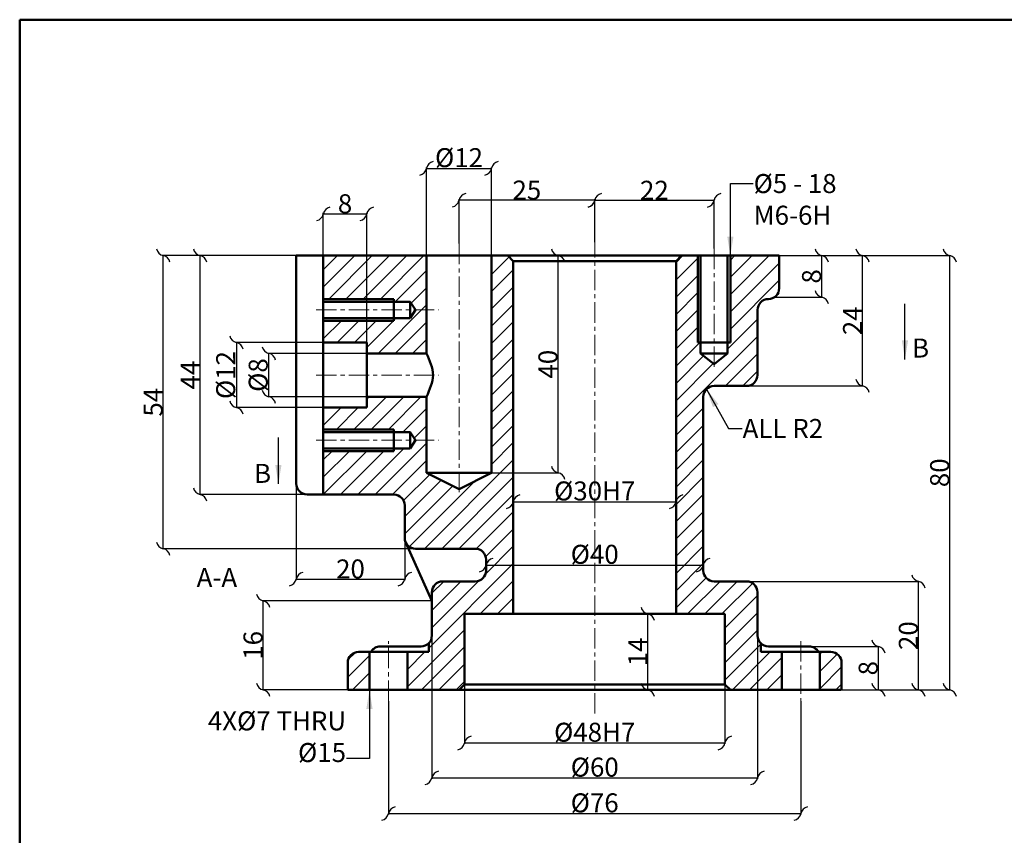
# Model space of a CAD drawing. Units: millimetres. Extents: x 10 to 373, y 9 to 285.
# Tile 2 of 3: x 10 to 191, y 135 to 285. Entities that reach past the tile are written whole.
import ezdxf

# ---------------------------------------------------------------- set-up
doc = ezdxf.new("R2010")
doc.units = ezdxf.units.MM
doc.header["$MEASUREMENT"] = 0
doc.linetypes.add('CENTER', pattern=[2, 1.25, -0.25, 0.25, -0.25])
for name, color, linetype, lineweight in [('M-CNTR', 1, 'CENTER', 18), ('M-DIMS', 2, 'Continuous', 25), ('M-HATC', 8, 'Continuous', 18), ('M-OUTL', 7, 'Continuous', 50), ('M-TEXT', 7, 'Continuous', 25), ('M-TTLB', 7, 'Continuous', 50)]:
    doc.layers.add(name, color=color, linetype=linetype, lineweight=lineweight)
doc.styles.get("Standard").update_dxf_attribs({"font": 'arial.ttf'})
doc.dimstyles.get("Standard").update_dxf_attribs({"dimtxt": 3.5, "dimasz": 3.5, "dimexe": 0.18, "dimexo": 0.0625, "dimgap": 0.09, "dimtad": 1, "dimdec": 0, "dimzin": 0, "dimdsep": 46, "dimtxsty": 'Standard', "dimblk": 'INTEGRAL', "dimcen": 0.09, "dimclre": 251, "dimadec": 0, "dimazin": 0, "dimtfac": 1, "dimtdec": 0, "dimtofl": 0, "dimtmove": 0, "dimatfit": 3, "dimfxl": 1, "dimtolj": 1, "dimtzin": 0, "dimarcsym": 0})

# ---------------------------------------------------------------- blocks, each defined once
blk = doc.blocks.new('_Integral')
at = {"color": 0, "linetype": 'ByBlock', "lineweight": -2}
for centre, start, end in [((0.445, -0.091), 102, 168), ((-0.445, 0.091), 282, 348)]:
    blk.add_arc(centre, 0.454, start, end, dxfattribs=at)
blk = doc.blocks.new('*D23')
at = {"layer": 'Defpoints', "color": 0, "transparency": 16777216}
for p in [(90.88, 252.1), (90.88, 244.06), (115.88, 244.35)]:
    blk.add_point(p, dxfattribs=at)
at = {"layer": 'M-DIMS', "color": 0, "lineweight": -2, "transparency": 16777216}
for p, q in [((90.88, 244.12), (90.88, 252.28)), ((115.88, 244.41), (115.88, 252.28)), ((115.88, 252.1), (90.88, 252.1))]:
    blk.add_line(p, q, dxfattribs=at)
at = {"layer": 'M-DIMS', "color": 0, "lineweight": -2, "transparency": 16777216, "xscale": 3.5, "yscale": 3.5, "zscale": 3.5, "rotation": 180}
blk.add_blockref('_Integral', (90.88, 252.1), dxfattribs=at)
at = {"layer": 'M-DIMS', "color": 0, "lineweight": -2, "transparency": 16777216, "xscale": 3.5, "yscale": 3.5, "zscale": 3.5}
blk.add_blockref('_Integral', (115.88, 252.1), dxfattribs=at)
at = {"layer": 'M-DIMS', "color": 0, "transparency": 16777216, "insert": (103.38, 253.98), "char_height": 3.5, "attachment_point": 5}
blk.add_mtext('\\A1;25', dxfattribs=at)
blk = doc.blocks.new('*D24')
at = {"layer": 'Defpoints', "color": 0, "transparency": 16777216}
for p in [(137.88, 252.09), (115.88, 244.35), (137.88, 243.16)]:
    blk.add_point(p, dxfattribs=at)
at = {"layer": 'M-DIMS', "color": 0, "lineweight": -2, "transparency": 16777216}
for p, q in [((115.88, 244.41), (115.88, 252.27)), ((137.88, 243.22), (137.88, 252.27)), ((115.88, 252.09), (137.88, 252.09))]:
    blk.add_line(p, q, dxfattribs=at)
at = {"layer": 'M-DIMS', "color": 0, "lineweight": -2, "transparency": 16777216, "xscale": 3.5, "yscale": 3.5, "zscale": 3.5, "rotation": 180}
blk.add_blockref('_Integral', (115.88, 252.09), dxfattribs=at)
at = {"layer": 'M-DIMS', "color": 0, "lineweight": -2, "transparency": 16777216, "xscale": 3.5, "yscale": 3.5, "zscale": 3.5}
blk.add_blockref('_Integral', (137.88, 252.09), dxfattribs=at)
at = {"layer": 'M-DIMS', "color": 0, "transparency": 16777216, "insert": (126.88, 253.94), "char_height": 3.5, "attachment_point": 5}
blk.add_mtext('\\A1;22', dxfattribs=at)
blk = doc.blocks.new('*D25')
at = {"layer": 'Defpoints', "color": 0, "transparency": 16777216}
for p in [(96.88, 257.98), (84.88, 241.9), (96.88, 241.9)]:
    blk.add_point(p, dxfattribs=at)
at = {"layer": 'M-DIMS', "color": 0, "lineweight": -2, "transparency": 16777216}
for p, q in [((84.88, 241.96), (84.88, 258.16)), ((84.88, 257.98), (96.88, 257.98)), ((96.88, 241.96), (96.88, 258.16))]:
    blk.add_line(p, q, dxfattribs=at)
at = {"layer": 'M-DIMS', "color": 0, "lineweight": -2, "transparency": 16777216, "xscale": 3.5, "yscale": 3.5, "zscale": 3.5, "rotation": 180}
blk.add_blockref('_Integral', (84.88, 257.98), dxfattribs=at)
at = {"layer": 'M-DIMS', "color": 0, "lineweight": -2, "transparency": 16777216, "xscale": 3.5, "yscale": 3.5, "zscale": 3.5}
blk.add_blockref('_Integral', (96.88, 257.98), dxfattribs=at)
at = {"layer": 'M-DIMS', "color": 0, "transparency": 16777216, "insert": (90.88, 259.95), "char_height": 3.5, "attachment_point": 5}
blk.add_mtext('\\A1;%%C12', dxfattribs=at)
blk = doc.blocks.new('*D26')
at = {"layer": 'Defpoints', "color": 0, "transparency": 16777216}
for p in [(73.88, 249.58), (65.88, 241.9), (73.88, 225.9)]:
    blk.add_point(p, dxfattribs=at)
at = {"layer": 'M-DIMS', "color": 0, "lineweight": -2, "transparency": 16777216}
for p, q in [((65.88, 241.96), (65.88, 249.76)), ((65.88, 249.58), (73.88, 249.58)), ((73.88, 225.96), (73.88, 249.76))]:
    blk.add_line(p, q, dxfattribs=at)
at = {"layer": 'M-DIMS', "color": 0, "lineweight": -2, "transparency": 16777216, "xscale": 3.5, "yscale": 3.5, "zscale": 3.5, "rotation": 180}
blk.add_blockref('_Integral', (65.88, 249.58), dxfattribs=at)
at = {"layer": 'M-DIMS', "color": 0, "lineweight": -2, "transparency": 16777216, "xscale": 3.5, "yscale": 3.5, "zscale": 3.5}
blk.add_blockref('_Integral', (73.88, 249.58), dxfattribs=at)
at = {"layer": 'M-DIMS', "color": 0, "transparency": 16777216, "insert": (69.88, 251.46), "char_height": 3.5, "attachment_point": 5}
blk.add_mtext('\\A1;8', dxfattribs=at)
blk = doc.blocks.new('*D27')
at = {"layer": 'Defpoints', "color": 0, "transparency": 16777216}
for p in [(55.86, 223.9), (73.88, 223.9), (73.88, 215.9)]:
    blk.add_point(p, dxfattribs=at)
at = {"layer": 'M-DIMS', "color": 0, "lineweight": -2, "transparency": 16777216}
for p, q in [((73.82, 223.9), (55.68, 223.9)), ((55.86, 215.9), (55.86, 223.9)), ((73.82, 215.9), (55.68, 215.9))]:
    blk.add_line(p, q, dxfattribs=at)
at = {"layer": 'M-DIMS', "color": 0, "lineweight": -2, "transparency": 16777216, "xscale": 3.5, "yscale": 3.5, "zscale": 3.5}
for p, rotation in [((55.86, 223.9), 90), ((55.86, 215.9), 270)]:
    blk.add_blockref('_Integral', p, dxfattribs=dict(at, rotation=rotation))
at = {"layer": 'M-DIMS', "color": 0, "transparency": 16777216, "insert": (53.88, 219.9), "char_height": 3.5, "attachment_point": 5, "rotation": 90}
blk.add_mtext('\\A1;%%C8', dxfattribs=at)
blk = doc.blocks.new('*D28')
at = {"layer": 'Defpoints', "color": 0, "transparency": 16777216}
for p in [(65.88, 225.9), (49.87, 213.9), (65.88, 213.9)]:
    blk.add_point(p, dxfattribs=at)
at = {"layer": 'M-DIMS', "color": 0, "lineweight": -2, "transparency": 16777216}
for p, q in [((65.82, 225.9), (49.69, 225.9)), ((49.87, 225.9), (49.87, 213.9)), ((65.82, 213.9), (49.69, 213.9))]:
    blk.add_line(p, q, dxfattribs=at)
at = {"layer": 'M-DIMS', "color": 0, "lineweight": -2, "transparency": 16777216, "xscale": 3.5, "yscale": 3.5, "zscale": 3.5}
for p, rotation in [((49.87, 225.9), 90), ((49.87, 213.9), 270)]:
    blk.add_blockref('_Integral', p, dxfattribs=dict(at, rotation=rotation))
at = {"layer": 'M-DIMS', "color": 0, "transparency": 16777216, "insert": (47.89, 219.9), "char_height": 3.5, "attachment_point": 5, "rotation": 90}
blk.add_mtext('\\A1;%%C12', dxfattribs=at)
blk = doc.blocks.new('*D29')
at = {"layer": 'Defpoints', "color": 0, "transparency": 16777216}
for p in [(43.17, 241.9), (60.88, 241.9), (62.88, 197.9)]:
    blk.add_point(p, dxfattribs=at)
at = {"layer": 'M-DIMS', "color": 0, "lineweight": -2, "transparency": 16777216}
for p, q in [((60.82, 241.9), (42.99, 241.9)), ((43.17, 197.9), (43.17, 241.9)), ((62.82, 197.9), (42.99, 197.9))]:
    blk.add_line(p, q, dxfattribs=at)
at = {"layer": 'M-DIMS', "color": 0, "lineweight": -2, "transparency": 16777216, "xscale": 3.5, "yscale": 3.5, "zscale": 3.5}
for p, rotation in [((43.17, 241.9), 90), ((43.17, 197.9), 270)]:
    blk.add_blockref('_Integral', p, dxfattribs=dict(at, rotation=rotation))
at = {"layer": 'M-DIMS', "color": 0, "transparency": 16777216, "insert": (41.33, 219.9), "char_height": 3.5, "attachment_point": 5, "rotation": 90}
blk.add_mtext('\\A1;44', dxfattribs=at)
blk = doc.blocks.new('*D30')
at = {"layer": 'Defpoints', "color": 0, "transparency": 16777216}
for p in [(36.39, 241.9), (60.88, 241.9), (82.88, 187.9)]:
    blk.add_point(p, dxfattribs=at)
at = {"layer": 'M-DIMS', "color": 0, "lineweight": -2, "transparency": 16777216}
for p, q in [((60.82, 241.9), (36.21, 241.9)), ((36.39, 187.9), (36.39, 241.9)), ((82.82, 187.9), (36.21, 187.9))]:
    blk.add_line(p, q, dxfattribs=at)
at = {"layer": 'M-DIMS', "color": 0, "lineweight": -2, "transparency": 16777216, "xscale": 3.5, "yscale": 3.5, "zscale": 3.5}
for p, rotation in [((36.39, 241.9), 90), ((36.39, 187.9), 270)]:
    blk.add_blockref('_Integral', p, dxfattribs=dict(at, rotation=rotation))
at = {"layer": 'M-DIMS', "color": 0, "transparency": 16777216, "insert": (34.52, 214.9), "char_height": 3.5, "attachment_point": 5, "rotation": 90}
blk.add_mtext('\\A1;54', dxfattribs=at)
blk = doc.blocks.new('*D31')
at = {"layer": 'Defpoints', "color": 0, "transparency": 16777216}
for p in [(60.88, 199.9), (80.88, 189.9), (80.88, 182.31)]:
    blk.add_point(p, dxfattribs=at)
at = {"layer": 'M-DIMS', "color": 0, "lineweight": -2, "transparency": 16777216}
for p, q in [((60.88, 199.84), (60.88, 182.13)), ((80.88, 189.84), (80.88, 182.13)), ((60.88, 182.31), (80.88, 182.31))]:
    blk.add_line(p, q, dxfattribs=at)
at = {"layer": 'M-DIMS', "color": 0, "lineweight": -2, "transparency": 16777216, "xscale": 3.5, "yscale": 3.5, "zscale": 3.5, "rotation": 180}
blk.add_blockref('_Integral', (60.88, 182.31), dxfattribs=at)
at = {"layer": 'M-DIMS', "color": 0, "lineweight": -2, "transparency": 16777216, "xscale": 3.5, "yscale": 3.5, "zscale": 3.5}
blk.add_blockref('_Integral', (80.88, 182.31), dxfattribs=at)
at = {"layer": 'M-DIMS', "color": 0, "transparency": 16777216, "insert": (70.88, 184.18), "char_height": 3.5, "attachment_point": 5}
blk.add_mtext('\\A1;20', dxfattribs=at)
blk = doc.blocks.new('*D32')
at = {"layer": 'Defpoints', "color": 0, "transparency": 16777216}
for p in [(54.8, 178.31), (85.88, 178.31), (70.38, 161.9)]:
    blk.add_point(p, dxfattribs=at)
at = {"layer": 'M-DIMS', "color": 0, "lineweight": -2, "transparency": 16777216}
for p, q in [((85.82, 178.31), (54.62, 178.31)), ((54.8, 161.9), (54.8, 178.31)), ((70.32, 161.9), (54.62, 161.9))]:
    blk.add_line(p, q, dxfattribs=at)
at = {"layer": 'M-DIMS', "color": 0, "lineweight": -2, "transparency": 16777216, "xscale": 3.5, "yscale": 3.5, "zscale": 3.5}
for p, rotation in [((54.8, 178.31), 90), ((54.8, 161.9), 270)]:
    blk.add_blockref('_Integral', p, dxfattribs=dict(at, rotation=rotation))
at = {"layer": 'M-DIMS', "color": 0, "transparency": 16777216, "insert": (52.92, 170.1), "char_height": 3.5, "attachment_point": 5, "rotation": 90}
blk.add_mtext('\\A1;16', dxfattribs=at)
blk = doc.blocks.new('*D33')
at = {"layer": 'Defpoints', "color": 0, "transparency": 16777216}
for p in [(149.88, 241.9), (157.72, 241.9), (149.01, 234.25)]:
    blk.add_point(p, dxfattribs=at)
at = {"layer": 'M-DIMS', "color": 0, "lineweight": -2, "transparency": 16777216}
for p, q in [((149.95, 241.9), (157.9, 241.9)), ((157.72, 234.25), (157.72, 241.9)), ((149.08, 234.25), (157.9, 234.25))]:
    blk.add_line(p, q, dxfattribs=at)
at = {"layer": 'M-DIMS', "color": 0, "lineweight": -2, "transparency": 16777216, "xscale": 3.5, "yscale": 3.5, "zscale": 3.5}
for p, rotation in [((157.72, 241.9), 90), ((157.72, 234.25), 270)]:
    blk.add_blockref('_Integral', p, dxfattribs=dict(at, rotation=rotation))
at = {"layer": 'M-DIMS', "color": 0, "transparency": 16777216, "insert": (155.84, 238.08), "char_height": 3.5, "attachment_point": 5, "rotation": 90}
blk.add_mtext('\\A1;8', dxfattribs=at)
blk = doc.blocks.new('*D34')
at = {"layer": 'Defpoints', "color": 0, "transparency": 16777216}
for p in [(149.88, 241.9), (165.24, 241.9), (143.88, 217.9)]:
    blk.add_point(p, dxfattribs=at)
at = {"layer": 'M-DIMS', "color": 0, "lineweight": -2, "transparency": 16777216}
for p, q in [((149.95, 241.9), (165.42, 241.9)), ((165.24, 217.9), (165.24, 241.9)), ((143.95, 217.9), (165.42, 217.9))]:
    blk.add_line(p, q, dxfattribs=at)
at = {"layer": 'M-DIMS', "color": 0, "lineweight": -2, "transparency": 16777216, "xscale": 3.5, "yscale": 3.5, "zscale": 3.5}
for p, rotation in [((165.24, 241.9), 90), ((165.24, 217.9), 270)]:
    blk.add_blockref('_Integral', p, dxfattribs=dict(at, rotation=rotation))
at = {"layer": 'M-DIMS', "color": 0, "transparency": 16777216, "insert": (163.39, 229.9), "char_height": 3.5, "attachment_point": 5, "rotation": 90}
blk.add_mtext('\\A1;24', dxfattribs=at)
blk = doc.blocks.new('*D35')
at = {"layer": 'Defpoints', "color": 0, "transparency": 16777216}
for p in [(155.38, 169.9), (168.15, 169.9), (161.38, 161.9)]:
    blk.add_point(p, dxfattribs=at)
at = {"layer": 'M-DIMS', "color": 0, "lineweight": -2, "transparency": 16777216}
for p, q in [((155.45, 169.9), (168.33, 169.9)), ((168.15, 161.9), (168.15, 169.9)), ((161.45, 161.9), (168.33, 161.9))]:
    blk.add_line(p, q, dxfattribs=at)
at = {"layer": 'M-DIMS', "color": 0, "lineweight": -2, "transparency": 16777216, "xscale": 3.5, "yscale": 3.5, "zscale": 3.5}
for p, rotation in [((168.15, 169.9), 90), ((168.15, 161.9), 270)]:
    blk.add_blockref('_Integral', p, dxfattribs=dict(at, rotation=rotation))
at = {"layer": 'M-DIMS', "color": 0, "transparency": 16777216, "insert": (166.27, 165.9), "char_height": 3.5, "attachment_point": 5, "rotation": 90}
blk.add_mtext('\\A1;8', dxfattribs=at)
blk = doc.blocks.new('*D36')
at = {"layer": 'Defpoints', "color": 0, "transparency": 16777216}
for p in [(137.88, 181.9), (175.54, 181.9), (161.38, 161.9)]:
    blk.add_point(p, dxfattribs=at)
at = {"layer": 'M-DIMS', "color": 0, "lineweight": -2, "transparency": 16777216}
for p, q in [((137.95, 181.9), (175.72, 181.9)), ((175.54, 161.9), (175.54, 181.9)), ((161.45, 161.9), (175.72, 161.9))]:
    blk.add_line(p, q, dxfattribs=at)
at = {"layer": 'M-DIMS', "color": 0, "lineweight": -2, "transparency": 16777216, "xscale": 3.5, "yscale": 3.5, "zscale": 3.5}
for p, rotation in [((175.54, 181.9), 90), ((175.54, 161.9), 270)]:
    blk.add_blockref('_Integral', p, dxfattribs=dict(at, rotation=rotation))
at = {"layer": 'M-DIMS', "color": 0, "transparency": 16777216, "insert": (173.67, 171.9), "char_height": 3.5, "attachment_point": 5, "rotation": 90}
blk.add_mtext('\\A1;20', dxfattribs=at)
blk = doc.blocks.new('*D37')
at = {"layer": 'Defpoints', "color": 0, "transparency": 16777216}
for p in [(149.88, 241.9), (181.31, 241.9), (161.38, 161.9)]:
    blk.add_point(p, dxfattribs=at)
at = {"layer": 'M-DIMS', "color": 0, "lineweight": -2, "transparency": 16777216}
for p, q in [((149.95, 241.9), (181.49, 241.9)), ((181.31, 161.9), (181.31, 241.9)), ((161.45, 161.9), (181.49, 161.9))]:
    blk.add_line(p, q, dxfattribs=at)
at = {"layer": 'M-DIMS', "color": 0, "lineweight": -2, "transparency": 16777216, "xscale": 3.5, "yscale": 3.5, "zscale": 3.5}
for p, rotation in [((181.31, 241.9), 90), ((181.31, 161.9), 270)]:
    blk.add_blockref('_Integral', p, dxfattribs=dict(at, rotation=rotation))
at = {"layer": 'M-DIMS', "color": 0, "transparency": 16777216, "insert": (179.44, 201.9), "char_height": 3.5, "attachment_point": 5, "rotation": 90}
blk.add_mtext('\\A1;80', dxfattribs=at)
blk = doc.blocks.new('*D38')
at = {"layer": 'Defpoints', "color": 0, "transparency": 16777216}
for p in [(125.66, 175.9), (125.66, 175.9), (125.66, 161.9)]:
    blk.add_point(p, dxfattribs=at)
at = {"layer": 'M-DIMS', "color": 0, "lineweight": -2, "transparency": 16777216}
for p, q in [((125.66, 161.9), (125.66, 175.9)), ((125.72, 175.9), (125.84, 175.9)), ((125.72, 161.9), (125.84, 161.9))]:
    blk.add_line(p, q, dxfattribs=at)
at = {"layer": 'M-DIMS', "color": 0, "lineweight": -2, "transparency": 16777216, "xscale": 3.5, "yscale": 3.5, "zscale": 3.5}
for p, rotation in [((125.66, 175.9), 90), ((125.66, 161.9), 270)]:
    blk.add_blockref('_Integral', p, dxfattribs=dict(at, rotation=rotation))
at = {"layer": 'M-DIMS', "color": 0, "transparency": 16777216, "insert": (123.81, 168.9), "char_height": 3.5, "attachment_point": 5, "rotation": 90}
blk.add_mtext('\\A1;14', dxfattribs=at)
blk = doc.blocks.new('*D39')
at = {"layer": 'Defpoints', "color": 0, "transparency": 16777216}
for p in [(91.88, 162.9), (139.88, 162.9), (139.88, 152.12)]:
    blk.add_point(p, dxfattribs=at)
at = {"layer": 'M-DIMS', "color": 0, "lineweight": -2, "transparency": 16777216}
for p, q in [((91.88, 162.84), (91.88, 151.94)), ((139.88, 162.84), (139.88, 151.94)), ((91.88, 152.12), (139.88, 152.12))]:
    blk.add_line(p, q, dxfattribs=at)
at = {"layer": 'M-DIMS', "color": 0, "lineweight": -2, "transparency": 16777216, "xscale": 3.5, "yscale": 3.5, "zscale": 3.5, "rotation": 180}
blk.add_blockref('_Integral', (91.88, 152.12), dxfattribs=at)
at = {"layer": 'M-DIMS', "color": 0, "lineweight": -2, "transparency": 16777216, "xscale": 3.5, "yscale": 3.5, "zscale": 3.5}
blk.add_blockref('_Integral', (139.88, 152.12), dxfattribs=at)
at = {"layer": 'M-DIMS', "color": 0, "transparency": 16777216, "insert": (115.88, 154.1), "char_height": 3.5, "attachment_point": 5}
blk.add_mtext('\\A1;%%C48H7', dxfattribs=at)
blk = doc.blocks.new('*D40')
at = {"layer": 'Defpoints', "color": 0, "transparency": 16777216}
for p in [(85.88, 171.9), (145.89, 171.81), (145.89, 145.69)]:
    blk.add_point(p, dxfattribs=at)
at = {"layer": 'M-DIMS', "color": 0, "lineweight": -2, "transparency": 16777216}
for p, q in [((85.88, 171.84), (85.88, 145.51)), ((145.89, 171.74), (145.89, 145.51)), ((85.88, 145.69), (145.89, 145.69))]:
    blk.add_line(p, q, dxfattribs=at)
at = {"layer": 'M-DIMS', "color": 0, "lineweight": -2, "transparency": 16777216, "xscale": 3.5, "yscale": 3.5, "zscale": 3.5, "rotation": 180}
blk.add_blockref('_Integral', (85.88, 145.69), dxfattribs=at)
at = {"layer": 'M-DIMS', "color": 0, "lineweight": -2, "transparency": 16777216, "xscale": 3.5, "yscale": 3.5, "zscale": 3.5}
blk.add_blockref('_Integral', (145.89, 145.69), dxfattribs=at)
at = {"layer": 'M-DIMS', "color": 0, "transparency": 16777216, "insert": (115.89, 147.67), "char_height": 3.5, "attachment_point": 5}
blk.add_mtext('\\A1;%%C60', dxfattribs=at)
blk = doc.blocks.new('*D41')
at = {"layer": 'Defpoints', "color": 0, "transparency": 16777216}
for p in [(77.88, 159.9), (153.88, 159.9), (153.88, 139.12)]:
    blk.add_point(p, dxfattribs=at)
at = {"layer": 'M-DIMS', "color": 0, "lineweight": -2, "transparency": 16777216}
for p, q in [((77.88, 159.84), (77.88, 138.94)), ((153.88, 159.84), (153.88, 138.94)), ((77.88, 139.12), (153.88, 139.12))]:
    blk.add_line(p, q, dxfattribs=at)
at = {"layer": 'M-DIMS', "color": 0, "lineweight": -2, "transparency": 16777216, "xscale": 3.5, "yscale": 3.5, "zscale": 3.5, "rotation": 180}
blk.add_blockref('_Integral', (77.88, 139.12), dxfattribs=at)
at = {"layer": 'M-DIMS', "color": 0, "lineweight": -2, "transparency": 16777216, "xscale": 3.5, "yscale": 3.5, "zscale": 3.5}
blk.add_blockref('_Integral', (153.88, 139.12), dxfattribs=at)
at = {"layer": 'M-DIMS', "color": 0, "transparency": 16777216, "insert": (115.88, 141.09), "char_height": 3.5, "attachment_point": 5}
blk.add_mtext('\\A1;%%C76', dxfattribs=at)
blk = doc.blocks.new('*D42')
at = {"layer": 'Defpoints', "color": 0, "transparency": 16777216}
for p in [(109.14, 241.9), (109.15, 241.9), (96.88, 201.9)]:
    blk.add_point(p, dxfattribs=at)
at = {"layer": 'M-DIMS', "color": 0, "lineweight": -2, "transparency": 16777216}
for p, q in [((109.15, 201.9), (109.15, 241.9)), ((109.2, 241.9), (109.33, 241.9)), ((96.95, 201.9), (109.33, 201.9))]:
    blk.add_line(p, q, dxfattribs=at)
at = {"layer": 'M-DIMS', "color": 0, "lineweight": -2, "transparency": 16777216, "xscale": 3.5, "yscale": 3.5, "zscale": 3.5}
for p, rotation in [((109.15, 241.9), 90), ((109.15, 201.9), 270)]:
    blk.add_blockref('_Integral', p, dxfattribs=dict(at, rotation=rotation))
at = {"layer": 'M-DIMS', "color": 0, "transparency": 16777216, "insert": (107.27, 221.9), "char_height": 3.5, "attachment_point": 5, "rotation": 90}
blk.add_mtext('\\A1;40', dxfattribs=at)
blk = doc.blocks.new('*D43')
at = {"layer": 'Defpoints', "color": 0, "transparency": 16777216}
for p in [(100.88, 196.57), (130.88, 196.57), (130.88, 196.57)]:
    blk.add_point(p, dxfattribs=at)
at = {"layer": 'M-DIMS', "color": 0, "lineweight": -2, "transparency": 16777216}
for p, q in [((100.88, 196.63), (100.88, 196.75)), ((100.88, 196.57), (130.88, 196.57)), ((130.88, 196.63), (130.88, 196.75))]:
    blk.add_line(p, q, dxfattribs=at)
at = {"layer": 'M-DIMS', "color": 0, "lineweight": -2, "transparency": 16777216, "xscale": 3.5, "yscale": 3.5, "zscale": 3.5, "rotation": 180}
blk.add_blockref('_Integral', (100.88, 196.57), dxfattribs=at)
at = {"layer": 'M-DIMS', "color": 0, "lineweight": -2, "transparency": 16777216, "xscale": 3.5, "yscale": 3.5, "zscale": 3.5}
blk.add_blockref('_Integral', (130.88, 196.57), dxfattribs=at)
at = {"layer": 'M-DIMS', "color": 0, "transparency": 16777216, "insert": (115.88, 198.55), "char_height": 3.5, "attachment_point": 5}
blk.add_mtext('\\A1;%%C30H7', dxfattribs=at)
blk = doc.blocks.new('*D44')
at = {"layer": 'Defpoints', "color": 0, "transparency": 16777216}
for p in [(95.88, 184.9), (135.88, 184.9), (135.88, 184.9)]:
    blk.add_point(p, dxfattribs=at)
at = {"layer": 'M-DIMS', "color": 0, "lineweight": -2, "transparency": 16777216}
for p, q in [((95.88, 184.96), (95.88, 185.08)), ((135.88, 184.96), (135.88, 185.08)), ((95.88, 184.9), (135.88, 184.9))]:
    blk.add_line(p, q, dxfattribs=at)
at = {"layer": 'M-DIMS', "color": 0, "lineweight": -2, "transparency": 16777216, "xscale": 3.5, "yscale": 3.5, "zscale": 3.5, "rotation": 180}
blk.add_blockref('_Integral', (95.88, 184.9), dxfattribs=at)
at = {"layer": 'M-DIMS', "color": 0, "lineweight": -2, "transparency": 16777216, "xscale": 3.5, "yscale": 3.5, "zscale": 3.5}
blk.add_blockref('_Integral', (135.88, 184.9), dxfattribs=at)
at = {"layer": 'M-DIMS', "color": 0, "transparency": 16777216, "insert": (115.88, 186.88), "char_height": 3.5, "attachment_point": 5}
blk.add_mtext('\\A1;%%C40', dxfattribs=at)
blk = doc.blocks.new('TAPPED-HOLE-M6')
for p, q in [((0, 4), (13, 4)), ((13, 0), (13, 4)), ((0, 3.5), (16, 3.5)), ((16, 0.5), (16, 3.5)), ((17, 2), (16, 3.5)), ((16, 0.5), (17, 2)), ((0, 0.5), (16, 0.5)), ((0, 0), (13, 0))]:
    blk.add_line(p, q)

msp = doc.modelspace()

# ---------------------------------------------------------------- hatches: boundary and pattern name
at = {"layer": 'M-HATC'}
h = msp.add_hatch(dxfattribs=at)
h.set_pattern_fill('ANSI31', color=256, scale=18)
h.set_pattern_definition([(45, (-376.4816, -107.6296), (-1.59099, 1.59099), [])])
h.paths.add_polyline_path([(84.88, 241.9), (65.88, 241.9), (65.88, 233.9), (78.88, 233.9), (78.88, 233.4), (81.88, 233.4), (82.88, 231.9), (84.88, 231.9)])
h.paths.add_polyline_path([(84.88, 231.9), (82.88, 231.9), (81.88, 230.4), (78.88, 230.4), (78.88, 229.9), (65.88, 229.9), (65.88, 225.9), (73.88, 225.9), (73.88, 223.9), (84.88, 223.9)])
h.paths.add_polyline_path([(84.88, 215.9), (73.88, 215.9), (73.88, 213.9), (65.88, 213.9), (65.88, 209.9), (78.88, 209.9), (78.88, 209.4), (81.88, 209.4), (82.88, 207.9), (84.88, 207.9)], flags=17)
h.paths.add_polyline_path([(90.88, 198.9), (84.88, 201.9), (84.88, 207.9), (82.88, 207.9), (81.88, 206.4), (78.88, 206.4), (78.88, 205.9), (65.88, 205.9), (65.88, 197.9), (78.88, 197.9, -0.414214), (80.88, 195.9), (80.88, 189.9, 0.414214), (82.88, 187.9), (93.88, 187.9, -0.414214), (95.88, 185.9), (95.88, 183.9, -0.414214), (93.88, 181.9), (87.88, 181.9, 0.414214), (85.88, 179.9), (85.88, 171.9, -0.198912), (85.3, 170.49), (85.3, 168.9), (81.38, 168.9), (81.38, 161.9), (90.88, 161.9), (91.88, 162.9), (91.88, 175.9), (100.88, 175.9), (100.88, 240.9), (99.88, 241.9), (96.88, 241.9), (96.88, 201.9)])
h.paths.add_polyline_path([(150.38, 168.9), (146.47, 168.9), (146.47, 170.49, -0.198912), (145.88, 171.9), (145.88, 179.9, 0.414214), (143.88, 181.9), (137.88, 181.9, -0.414214), (135.88, 183.9), (135.88, 215.9, -0.414214), (137.88, 217.9), (143.88, 217.9, 0.414214), (145.88, 219.9), (145.88, 231.9, -0.414214), (147.88, 233.9, 0.414214), (149.88, 235.9), (149.88, 241.9), (140.88, 241.9), (140.88, 225.9), (140.38, 225.9), (140.38, 223.9), (137.88, 221.9), (135.38, 223.9), (135.38, 225.9), (134.88, 225.9), (134.88, 241.9), (131.88, 241.9), (130.88, 240.9), (130.88, 175.9), (139.88, 175.9), (139.88, 162.9), (140.88, 161.9), (150.38, 161.9)])
edge = h.paths.add_edge_path()
edge.add_arc((72.38, 166.9), 2, 90, 180)
edge.add_line((70.38, 166.9), (70.38, 161.9))
edge.add_line((70.38, 161.9), (74.38, 161.9))
edge.add_line((74.38, 161.9), (74.38, 168.9))
edge.add_line((74.38, 168.9), (72.38, 168.9))
edge = h.paths.add_edge_path()
edge.add_arc((159.38, 166.9), 2, 360, 450)
edge.add_line((159.38, 168.9), (157.38, 168.9))
edge.add_line((157.38, 168.9), (157.38, 161.9))
edge.add_line((157.38, 161.9), (161.38, 161.9))
edge.add_line((161.38, 161.9), (161.38, 166.9))

# ---------------------------------------------------------------- linework, layer by layer
at = {"layer": 'M-CNTR', "ltscale": 3}
for p, q in [((90.88, 244.06), (90.88, 197.49)), ((115.88, 157.55), (115.88, 244.35)), ((137.88, 243.16), (137.88, 221.41)), ((64.57, 231.9), (87.14, 231.9)), ((64.57, 219.9), (87.14, 219.9)), ((64.57, 207.9), (87.14, 207.9)), ((77.88, 159.9), (77.88, 170.9)), ((153.88, 170.9), (153.88, 159.9))]:
    msp.add_line(p, q, dxfattribs=at)
at = {"layer": 'M-OUTL'}
for p, q in [((60.88, 241.9), (149.88, 241.9)), ((60.88, 241.9), (60.88, 199.9)), ((65.88, 197.9), (65.88, 241.9)), ((84.88, 223.9), (84.88, 241.9)), ((96.88, 201.9), (96.88, 241.9)), ((99.88, 241.9), (100.88, 240.9)), ((130.88, 240.9), (131.88, 241.9)), ((134.88, 241.9), (134.88, 225.9)), ((135.38, 241.9), (135.38, 223.9)), ((140.38, 241.9), (140.38, 223.9)), ((140.88, 241.9), (140.88, 225.9)), ((149.88, 241.9), (149.88, 235.9)), ((100.88, 175.9), (100.88, 240.9)), ((100.88, 240.9), (130.88, 240.9)), ((130.88, 175.9), (130.88, 240.9)), ((147.88, 233.9), (147.88, 233.9)), ((145.88, 219.9), (145.88, 231.9)), ((65.88, 225.9), (73.88, 225.9)), ((73.88, 213.9), (73.88, 225.9)), ((134.88, 225.9), (140.88, 225.9)), ((73.88, 223.9), (84.88, 223.9)), ((135.38, 223.9), (140.38, 223.9)), ((135.38, 223.9), (137.88, 221.9)), ((137.88, 221.9), (140.38, 223.9)), ((137.88, 217.9), (143.88, 217.9)), ((73.88, 215.9), (84.88, 215.9)), ((84.88, 201.9), (84.88, 215.9)), ((135.88, 183.9), (135.88, 215.9)), ((65.88, 213.9), (73.88, 213.9)), ((84.88, 201.9), (96.88, 201.9)), ((84.88, 201.9), (90.88, 198.9)), ((90.88, 198.9), (96.88, 201.9)), ((62.88, 197.9), (78.88, 197.9)), ((80.88, 195.9), (80.88, 189.9)), ((85.88, 178.31), (81.11, 188.97)), ((82.88, 187.9), (93.88, 187.9)), ((95.88, 183.9), (95.88, 185.9)), ((93.88, 181.9), (87.88, 181.9)), ((137.88, 181.9), (143.88, 181.9)), ((85.88, 171.9), (85.88, 179.9)), ((145.88, 179.9), (145.88, 171.9)), ((91.88, 162.9), (91.88, 175.9)), ((91.88, 175.9), (139.88, 175.9)), ((139.88, 162.9), (139.88, 175.9)), ((72.38, 168.9), (85.3, 168.9)), ((74.38, 161.9), (74.38, 168.9)), ((76.38, 169.9), (83.88, 169.9)), ((81.38, 161.9), (81.38, 168.9)), ((85.3, 170.49), (85.3, 168.9)), ((146.47, 170.49), (146.47, 168.9)), ((146.47, 168.9), (159.38, 168.9)), ((155.38, 169.9), (147.88, 169.9)), ((150.38, 168.9), (150.38, 161.9)), ((157.38, 168.9), (157.38, 161.9)), ((70.38, 161.9), (70.38, 166.9)), ((161.38, 161.9), (161.38, 166.9)), ((70.38, 161.9), (161.38, 161.9)), ((90.88, 161.9), (91.88, 162.9)), ((91.88, 162.9), (139.88, 162.9)), ((139.88, 162.9), (140.88, 161.9))]:
    msp.add_line(p, q, dxfattribs=at)
for centre, start, end in [((147.88, 235.9), 270, 0), ((147.88, 231.9), 90, 180), ((143.88, 219.9), 270, 0), ((137.88, 215.9), 90, 180), ((62.88, 199.9), 180, 270), ((78.88, 195.9), 0, 90), ((82.88, 189.9), 180, 270), ((93.88, 185.9), 0, 90), ((93.88, 183.9), 270, 0), ((137.88, 183.9), 180, 270), ((87.88, 179.9), 90, 180), ((143.88, 179.9), 0, 90), ((83.88, 171.9), 270, 0), ((147.88, 171.9), 180, 270), ((72.38, 166.9), 90, 180), ((76.38, 167.9), 90, 150), ((155.38, 167.9), 30, 90), ((159.38, 166.9), 0, 90)]:
    msp.add_arc(centre, 2, start, end, dxfattribs=at)
msp.add_open_spline([(84.88, 223.9), (85.49, 222.57), (86.69, 219.9), (85.49, 217.24), (84.88, 215.9)], degree=3, dxfattribs=at)
at = {"layer": 'M-TTLB'}
msp.add_lwpolyline([(9.93, 285.37), (372.77, 285.37), (372.77, 8.8), (9.93, 8.8)], close=True, dxfattribs=at)

# ---------------------------------------------------------------- block references
at = {"layer": 'M-OUTL'}
for p in [(65.89, 229.9), (65.89, 205.9)]:
    msp.add_blockref('TAPPED-HOLE-M6', p, dxfattribs=at)

# ---------------------------------------------------------------- texts
at = {"layer": 'M-TEXT', "char_height": 3.5}
for s, insert, attachment_point in [('%%C5 - 18 \\PM6-6H ', (145.16, 256.93), 1), ('\\A1;B', (175.93, 224.88), 5), ('ALL R2', (143.13, 211.81), 1), ('\\A1;B', (54.69, 201.79), 5), ('\\A1;A-A', (46.27, 182.61), 5), ('4X%%C7 THRU\\P%%C15', (70.06, 147.52), 9)]:
    msp.add_mtext(s, dxfattribs=dict(at, insert=insert, attachment_point=attachment_point))

# ---------------------------------------------------------------- dimensions: what is measured, and where the dimension line sits
at = {"layer": 'M-DIMS'}
for base, p1, p2, text, picture, middle in [((96.88, 257.98), (84.88, 241.9), (96.88, 241.9), '%%C<>', '*D25', (90.88, 259.95)), ((130.88, 196.57), (100.88, 196.57), (130.88, 196.57), '%%C<>H7', '*D43', (115.88, 198.55)), ((135.88, 184.9), (95.88, 184.9), (135.88, 184.9), '%%C<>', '*D44', (115.88, 186.88)), ((145.89, 145.69), (85.88, 171.9), (145.89, 171.81), '%%C<>', '*D40', (115.89, 147.67)), ((139.88, 152.12), (91.88, 162.9), (139.88, 162.9), '%%C<>H7', '*D39', (115.88, 154.1)), ((153.88, 139.12), (77.88, 159.9), (153.88, 159.9), '%%C<>', '*D41', (115.88, 141.09))]:
    dim = msp.add_linear_dim(base=base, p1=p1, p2=p2, text=text, dimstyle='Standard', override={"dimclrd": 0, "dimclre": 0, "dimclrt": 0}, dxfattribs=at)
    dim.commit()
    dim.dimension.update_dxf_attribs({"geometry": picture, "text_midpoint": middle})
for base, p1, p2, picture, middle in [((90.88, 252.1), (115.88, 244.35), (90.88, 244.06), '*D23', (103.38, 253.98)), ((137.88, 252.09), (115.88, 244.35), (137.88, 243.16), '*D24', (126.88, 253.94)), ((73.88, 249.58), (65.88, 241.9), (73.88, 225.9), '*D26', (69.88, 251.46)), ((80.88, 182.31), (60.88, 199.9), (80.88, 189.9), '*D31', (70.88, 184.18))]:
    dim = msp.add_linear_dim(base=base, p1=p1, p2=p2, dimstyle='Standard', override={"dimclrd": 0, "dimclre": 0, "dimclrt": 0}, dxfattribs=at)
    dim.commit()
    dim.dimension.update_dxf_attribs({"geometry": picture, "text_midpoint": middle})
for base, p1, p2, picture, middle in [((36.39, 241.9), (82.88, 187.9), (60.88, 241.9), '*D30', (34.52, 214.9)), ((43.17, 241.9), (62.88, 197.9), (60.88, 241.9), '*D29', (41.33, 219.9)), ((109.15, 241.9), (96.88, 201.9), (109.14, 241.9), '*D42', (107.27, 221.9)), ((165.24, 241.9), (143.88, 217.9), (149.88, 241.9), '*D34', (163.39, 229.9)), ((157.72, 241.9), (149.01, 234.25), (149.88, 241.9), '*D33', (155.84, 238.08)), ((181.31, 241.9), (161.38, 161.9), (149.88, 241.9), '*D37', (179.44, 201.9)), ((175.54, 181.9), (161.38, 161.9), (137.88, 181.9), '*D36', (173.67, 171.9)), ((54.8, 178.31), (70.38, 161.9), (85.88, 178.31), '*D32', (52.92, 170.1)), ((125.66, 175.9), (125.66, 161.9), (125.66, 175.9), '*D38', (123.81, 168.9)), ((168.15, 169.9), (161.38, 161.9), (155.38, 169.9), '*D35', (166.27, 165.9))]:
    dim = msp.add_linear_dim(base=base, p1=p1, p2=p2, angle=90, dimstyle='Standard', override={"dimclrd": 0, "dimclre": 0, "dimclrt": 0}, dxfattribs=at)
    dim.commit()
    dim.dimension.update_dxf_attribs({"geometry": picture, "text_midpoint": middle})
for base, p1, p2, picture, middle in [((49.87, 213.9), (65.88, 225.9), (65.88, 213.9), '*D28', (47.89, 219.9)), ((55.86, 223.9), (73.88, 215.9), (73.88, 223.9), '*D27', (53.88, 219.9))]:
    dim = msp.add_linear_dim(base=base, p1=p1, p2=p2, angle=90, text='%%C<>', dimstyle='Standard', override={"dimclrd": 0, "dimclre": 0, "dimclrt": 0}, dxfattribs=at)
    dim.commit()
    dim.dimension.update_dxf_attribs({"geometry": picture, "text_midpoint": middle})

# ---------------------------------------------------------------- leaders
at = {"layer": 'M-DIMS', "annotation_type": 0, "has_hookline": 1, "hookline_direction": 1}
for points, text_width in [([(140.88, 241.9), (140.88, 255.18), (145.07, 255.18)], 15.89), ([(136.47, 217.32), (140.52, 210.06), (143.04, 210.06)], 16.05), ([(74.38, 161.9), (74.38, 149.27), (70.15, 149.27)], 26.99)]:
    msp.add_leader(points, dimstyle='Standard', override={"dimgap": 0.09, "dimtad": 0}, dxfattribs=dict(at, text_width=text_width))
at = {"layer": 'M-DIMS'}
for points in [[(173.05, 222.79), (173.05, 233.04)], [(57.6, 199.85), (57.6, 208.39)]]:
    msp.add_leader(points, dimstyle='Standard', override={"dimgap": 0.09, "dimtad": 0}, dxfattribs=at)

doc.saveas('drawing.dxf')
